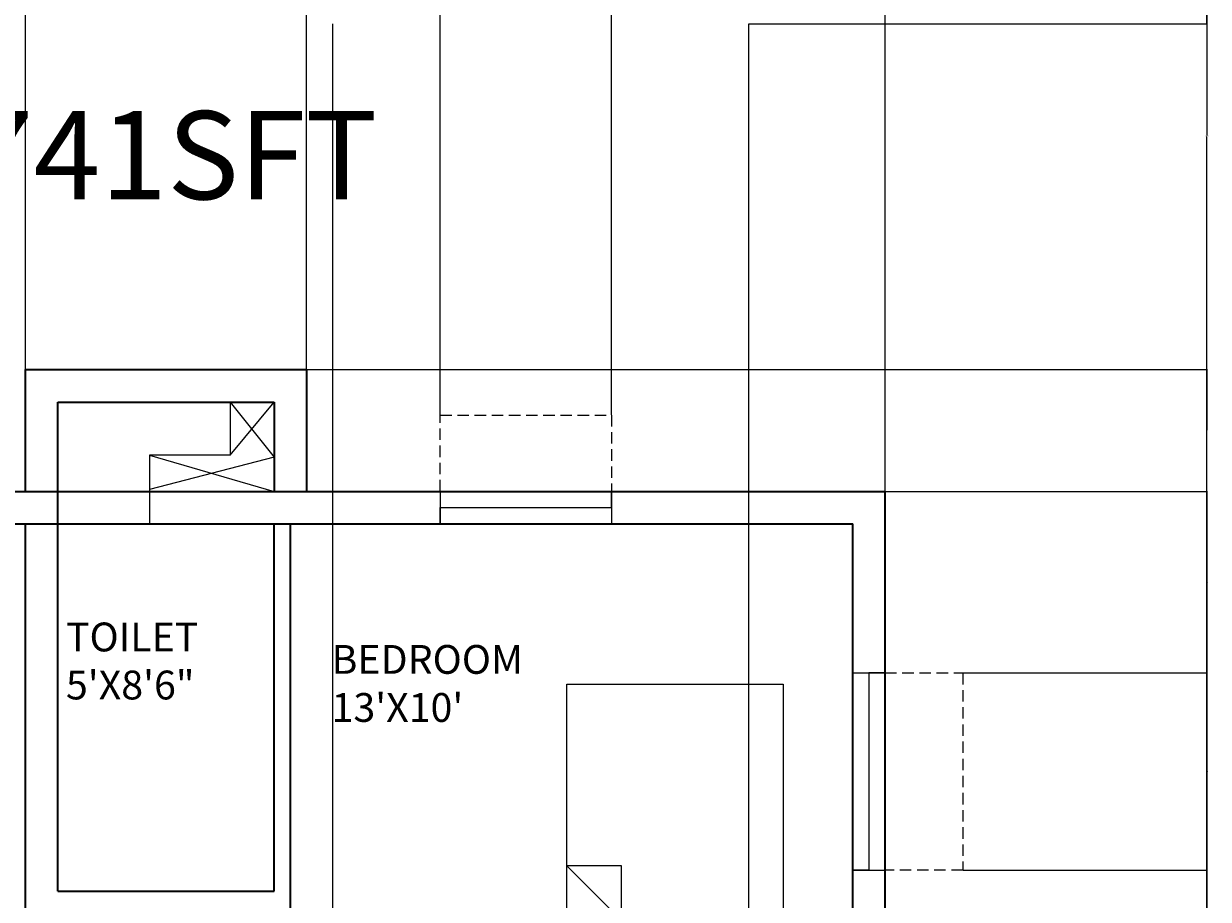
# Model space of a CAD drawing. Units: inches. Extents: x 276 to 912, y -567 to 621.
# Tile 4 of 7: x 583 to 912, y -178 to 65. Entities that reach past the tile are written whole.
import ezdxf

# ---------------------------------------------------------------- set-up
doc = ezdxf.new("R2010")
doc.units = ezdxf.units.IN
doc.linetypes.add('HIDDEN2', pattern=[4.7625, 3.175, -1.5875])
for name, color, linetype, lineweight in [('A-ANNO-DIMS', 2, 'Continuous', 18), ('A-ANNO-TEXT', 7, 'Continuous', 35), ('A-AREA-IDEN', 7, 'Continuous', 18), ('A-FLOR-OVHD', 8, 'HIDDEN2', 13), ('A-FLOR-SHFT', 8, 'Continuous', 18), ('A-FURN', 8, 'Continuous', 18), ('A-GLAZ', 4, 'Continuous', 18), ('A-WALL', 7, 'Continuous', 35)]:
    doc.layers.add(name, color=color, linetype=linetype, lineweight=lineweight)
doc.dimstyles.get("Standard").update_dxf_attribs({"dimtxt": 0.18, "dimasz": 0.18, "dimexe": 0.18, "dimexo": 0.0625, "dimgap": 0.09, "dimtad": 0, "dimtih": 1, "dimtoh": 1, "dimdec": 4, "dimzin": 0, "dimdsep": 46, "dimtxsty": 'Standard', "dimcen": 0.09, "dimadec": 0, "dimazin": 0, "dimtfac": 1, "dimtdec": 4, "dimtofl": 0, "dimtmove": 0, "dimatfit": 3, "dimfxl": 1, "dimtolj": 1, "dimtzin": 0, "dimarcsym": 0})

# ---------------------------------------------------------------- blocks, each defined once
blk = doc.blocks.new('Bed - Queen')
for p, q in [((0, -80.00003), (0, 0)), ((0, 0), (59.99999, 0)), ((59.99999, 0), (59.99999, -80.00003)), ((7.99999, -1.2), (28.79998, -1.2)), ((7.99999, -14.4), (7.99999, -1.2)), ((28.79998, -1.2), (28.79998, -14.4)), ((31.19999, -1.2), (51.99999, -1.2)), ((31.19999, -14.4), (31.19999, -1.2)), ((51.99999, -1.2), (51.99999, -16.4)), ((0, -14.4), (44.8, -14.4)), ((59.99999, -29.6), (44.8, -14.4)), ((44.8, -14.4), (44.8, -29.6)), ((51.99999, -16.4), (46.79936, -16.4)), ((44.8, -16.8), (0, -16.8)), ((44.8, -29.6), (59.99999, -29.6)), ((59.99999, -80.00003), (0, -80.00003))]:
    blk.add_line(p, q)
blk = doc.blocks.new('*D24')
at = {"layer": 'A-ANNO-DIMS', "color": 0, "lineweight": -2, "transparency": 16777216}
for p, q in [((333.082179, 103.255751), (333.082179, -553.223061)), ((854.209085, -327.604004), (854.209085, -553.223061)), ((333.262179, -553.043061), (593.255632, -553.043061)), ((854.029085, -553.043061), (594.035632, -553.043061))]:
    blk.add_line(p, q, dxfattribs=at)
at = {"layer": 'A-ANNO-DIMS', "color": 0, "transparency": 16777216}
for points in [[(333.262179, -553.013061), (333.262179, -553.073061), (333.082179, -553.043061)], [(854.029085, -553.013061), (854.029085, -553.073061), (854.209085, -553.043061)]]:
    blk.add_solid(points, dxfattribs=at)
at = {"layer": 'Defpoints', "color": 0, "transparency": 16777216}
for p in [(333.082179, 103.318251), (854.209085, -327.541504), (854.209085, -553.043061)]:
    blk.add_point(p, dxfattribs=at)
at = {"layer": 'A-ANNO-DIMS', "color": 0, "transparency": 16777216, "insert": (593.645632, -553.043061), "char_height": 0.18, "attachment_point": 5}
blk.add_mtext('\\A1;521.1', dxfattribs=at)
blk = doc.blocks.new('*D25')
at = {"layer": 'A-ANNO-DIMS', "color": 0, "lineweight": -2, "transparency": 16777216}
for p, q in [((478.5, 564.29), (911.39, 564.29)), ((911.21, 564.11), (911.21, 34.31)), ((911.21, -495.86), (911.21, 33.95)), ((582.98, -496.04), (911.39, -496.04))]:
    blk.add_line(p, q, dxfattribs=at)
at = {"layer": 'A-ANNO-DIMS', "color": 0, "transparency": 16777216}
for points in [[(911.18, 564.11), (911.24, 564.11), (911.21, 564.29)], [(911.18, -495.86), (911.24, -495.86), (911.21, -496.04)]]:
    blk.add_solid(points, dxfattribs=at)
at = {"layer": 'Defpoints', "color": 0, "transparency": 16777216}
for p in [(478.44, 564.29), (582.92, -496.04), (911.21, -496.04)]:
    blk.add_point(p, dxfattribs=at)
at = {"layer": 'A-ANNO-DIMS', "color": 0, "transparency": 16777216, "insert": (911.21, 34.13), "char_height": 0.18, "attachment_point": 5}
blk.add_mtext('\\A1;1060.3', dxfattribs=at)
blk = doc.blocks.new('*D33')
at = {"layer": 'A-ANNO-DIMS', "color": 0, "lineweight": -2, "transparency": 16777216}
for p, q in [((553.582179, 65.246155), (553.582179, -553.223061)), ((668.582179, 65.246155), (668.582179, -553.223061)), ((553.762179, -553.043061), (610.812179, -553.043061)), ((668.402179, -553.043061), (611.352179, -553.043061))]:
    blk.add_line(p, q, dxfattribs=at)
at = {"layer": 'A-ANNO-DIMS', "color": 0, "transparency": 16777216}
for points in [[(553.762179, -553.013061), (553.762179, -553.073061), (553.582179, -553.043061)], [(668.402179, -553.013061), (668.402179, -553.073061), (668.582179, -553.043061)]]:
    blk.add_solid(points, dxfattribs=at)
at = {"layer": 'Defpoints', "color": 0, "transparency": 16777216}
for p in [(553.582179, 65.308655), (668.582179, 65.308655), (668.582179, -553.043061)]:
    blk.add_point(p, dxfattribs=at)
at = {"layer": 'A-ANNO-DIMS', "color": 0, "transparency": 16777216, "insert": (611.082179, -553.043061), "char_height": 0.18, "attachment_point": 5}
blk.add_mtext('\\A1;115', dxfattribs=at)
blk = doc.blocks.new('*D34')
at = {"layer": 'A-ANNO-DIMS', "color": 0, "lineweight": -2, "transparency": 16777216}
for p, q in [((668.58, 65.25), (668.58, -553.22)), ((784, 65.25), (784, -553.22)), ((668.76, -553.04), (725.81, -553.04)), ((783.82, -553.04), (726.77, -553.04))]:
    blk.add_line(p, q, dxfattribs=at)
at = {"layer": 'A-ANNO-DIMS', "color": 0, "transparency": 16777216}
for points in [[(668.76, -553.01), (668.76, -553.07), (668.58, -553.04)], [(783.82, -553.01), (783.82, -553.07), (784, -553.04)]]:
    blk.add_solid(points, dxfattribs=at)
at = {"layer": 'Defpoints', "color": 0, "transparency": 16777216}
for p in [(668.58, 65.31), (784, 65.31), (784, -553.04)]:
    blk.add_point(p, dxfattribs=at)
at = {"layer": 'A-ANNO-DIMS', "color": 0, "transparency": 16777216, "insert": (726.29, -553.04), "char_height": 0.18, "attachment_point": 5}
blk.add_mtext('\\A1;115.42', dxfattribs=at)
blk = doc.blocks.new('*D35')
at = {"layer": 'A-ANNO-DIMS', "color": 0, "lineweight": -2, "transparency": 16777216}
for p, q in [((784.0623, 103.318251), (911.389085, 103.318251)), ((911.209085, 103.138251), (911.209085, 84.493453)), ((911.209085, 65.488655), (911.209085, 84.133453)), ((784.0623, 65.308655), (911.389085, 65.308655))]:
    blk.add_line(p, q, dxfattribs=at)
at = {"layer": 'A-ANNO-DIMS', "color": 0, "transparency": 16777216}
for points in [[(911.179085, 103.138251), (911.239085, 103.138251), (911.209085, 103.318251)], [(911.179085, 65.488655), (911.239085, 65.488655), (911.209085, 65.308655)]]:
    blk.add_solid(points, dxfattribs=at)
at = {"layer": 'Defpoints', "color": 0, "transparency": 16777216}
for p in [(783.9998, 103.318251), (911.209085, 103.318251), (783.9998, 65.308655)]:
    blk.add_point(p, dxfattribs=at)
at = {"layer": 'A-ANNO-DIMS', "color": 0, "transparency": 16777216, "insert": (911.209085, 84.313453), "char_height": 0.18, "attachment_point": 5}
blk.add_mtext('\\A1;38.01', dxfattribs=at)
blk = doc.blocks.new('*D54')
at = {"layer": 'A-ANNO-DIMS', "color": 0, "lineweight": -2, "transparency": 16777216}
for p, q in [((821.980989, -64.541504), (911.389085, -64.541504)), ((911.209085, -64.721504), (911.209085, -259.361504)), ((911.209085, -454.361504), (911.209085, -259.721504)), ((821.980989, -454.541504), (911.389085, -454.541504))]:
    blk.add_line(p, q, dxfattribs=at)
at = {"layer": 'A-ANNO-DIMS', "color": 0, "transparency": 16777216}
for points in [[(911.179085, -64.721504), (911.239085, -64.721504), (911.209085, -64.541504)], [(911.179085, -454.361504), (911.239085, -454.361504), (911.209085, -454.541504)]]:
    blk.add_solid(points, dxfattribs=at)
at = {"layer": 'Defpoints', "color": 0, "transparency": 16777216}
for p in [(821.918489, -64.541504), (821.918489, -454.541504), (911.209085, -454.541504)]:
    blk.add_point(p, dxfattribs=at)
at = {"layer": 'A-ANNO-DIMS', "color": 0, "transparency": 16777216, "insert": (911.209085, -259.541504), "char_height": 0.18, "attachment_point": 5}
blk.add_mtext('\\A1;390', dxfattribs=at)
blk = doc.blocks.new('*D59')
at = {"layer": 'A-ANNO-DIMS', "color": 0, "lineweight": -2, "transparency": 16777216}
for p, q in [((333.082179, -81.315568), (333.082179, 621.473746)), ((333.262179, 621.293746), (457.725334, 621.293746)), ((583.238489, 621.293746), (458.775334, 621.293746)), ((583.418489, -30.671128), (583.418489, 621.473746))]:
    blk.add_line(p, q, dxfattribs=at)
at = {"layer": 'A-ANNO-DIMS', "color": 0, "transparency": 16777216}
for points in [[(333.262179, 621.323746), (333.262179, 621.263746), (333.082179, 621.293746)], [(583.238489, 621.323746), (583.238489, 621.263746), (583.418489, 621.293746)]]:
    blk.add_solid(points, dxfattribs=at)
at = {"layer": 'Defpoints', "color": 0, "transparency": 16777216}
for p in [(583.418489, 621.293746), (583.418489, -30.733628), (333.082179, -81.378068)]:
    blk.add_point(p, dxfattribs=at)
at = {"layer": 'A-ANNO-DIMS', "color": 0, "transparency": 16777216, "insert": (458.250334, 621.293746), "char_height": 0.18, "attachment_point": 5}
blk.add_mtext('\\A1;250.34', dxfattribs=at)
blk = doc.blocks.new('*D60')
at = {"layer": 'A-ANNO-DIMS', "color": 0, "lineweight": -2, "transparency": 16777216}
for p, q in [((583.418489, -30.671128), (583.418489, 621.473746)), ((583.598489, 621.293746), (622.178489, 621.293746)), ((661.238489, 621.293746), (622.658489, 621.293746)), ((661.418489, -30.671128), (661.418489, 621.473746))]:
    blk.add_line(p, q, dxfattribs=at)
at = {"layer": 'A-ANNO-DIMS', "color": 0, "transparency": 16777216}
for points in [[(583.598489, 621.323746), (583.598489, 621.263746), (583.418489, 621.293746)], [(661.238489, 621.323746), (661.238489, 621.263746), (661.418489, 621.293746)]]:
    blk.add_solid(points, dxfattribs=at)
at = {"layer": 'Defpoints', "color": 0, "transparency": 16777216}
for p in [(661.418489, 621.293746), (583.418489, -30.733628), (661.418489, -30.733628)]:
    blk.add_point(p, dxfattribs=at)
at = {"layer": 'A-ANNO-DIMS', "color": 0, "transparency": 16777216, "insert": (622.418489, 621.293746), "char_height": 0.18, "attachment_point": 5}
blk.add_mtext('\\A1;78', dxfattribs=at)
blk = doc.blocks.new('*D61')
at = {"layer": 'A-ANNO-DIMS', "color": 0, "lineweight": -2, "transparency": 16777216}
for p, q in [((661.418489, -30.671128), (661.418489, 621.473746)), ((661.598489, 621.293746), (741.263489, 621.293746)), ((821.738489, 621.293746), (742.073489, 621.293746)), ((821.918489, -64.479004), (821.918489, 621.473746))]:
    blk.add_line(p, q, dxfattribs=at)
at = {"layer": 'A-ANNO-DIMS', "color": 0, "transparency": 16777216}
for points in [[(661.598489, 621.323746), (661.598489, 621.263746), (661.418489, 621.293746)], [(821.738489, 621.323746), (821.738489, 621.263746), (821.918489, 621.293746)]]:
    blk.add_solid(points, dxfattribs=at)
at = {"layer": 'Defpoints', "color": 0, "transparency": 16777216}
for p in [(821.918489, 621.293746), (661.418489, -30.733628), (821.918489, -64.541504)]:
    blk.add_point(p, dxfattribs=at)
at = {"layer": 'A-ANNO-DIMS', "color": 0, "transparency": 16777216, "insert": (741.668489, 621.293746), "char_height": 0.18, "attachment_point": 5}
blk.add_mtext('\\A1;160.5', dxfattribs=at)
blk = doc.blocks.new('*D62')
at = {"layer": 'A-ANNO-DIMS', "color": 0, "lineweight": -2, "transparency": 16777216}
for p, q in [((661.480989, -30.733628), (911.389085, -30.733628)), ((911.209085, -30.913628), (911.209085, -47.457566)), ((911.209085, -64.361504), (911.209085, -47.817566)), ((661.480989, -64.541504), (911.389085, -64.541504))]:
    blk.add_line(p, q, dxfattribs=at)
at = {"layer": 'A-ANNO-DIMS', "color": 0, "transparency": 16777216}
for points in [[(911.179085, -30.913628), (911.239085, -30.913628), (911.209085, -30.733628)], [(911.179085, -64.361504), (911.239085, -64.361504), (911.209085, -64.541504)]]:
    blk.add_solid(points, dxfattribs=at)
at = {"layer": 'Defpoints', "color": 0, "transparency": 16777216}
for p in [(661.418489, -30.733628), (661.418489, -64.541504), (911.209085, -64.541504)]:
    blk.add_point(p, dxfattribs=at)
at = {"layer": 'A-ANNO-DIMS', "color": 0, "transparency": 16777216, "insert": (911.209085, -47.637566), "char_height": 0.18, "attachment_point": 5}
blk.add_mtext('\\A1;33.81', dxfattribs=at)
blk = doc.blocks.new('*D72')
at = {"layer": 'A-ANNO-DIMS', "color": 0, "lineweight": -2, "transparency": 16777216}
for p, q in [((698.51, -43.28), (698.51, 621.47)), ((698.69, 621.29), (721.9, 621.29)), ((745.83, 621.29), (722.62, 621.29)), ((746.01, -43.28), (746.01, 621.47))]:
    blk.add_line(p, q, dxfattribs=at)
at = {"layer": 'A-ANNO-DIMS', "color": 0, "transparency": 16777216}
for points in [[(698.69, 621.32), (698.69, 621.26), (698.51, 621.29)], [(745.83, 621.32), (745.83, 621.26), (746.01, 621.29)]]:
    blk.add_solid(points, dxfattribs=at)
at = {"layer": 'Defpoints', "color": 0, "transparency": 16777216}
for p in [(746.01, 621.29), (698.51, -43.34), (746.01, -43.34)]:
    blk.add_point(p, dxfattribs=at)
at = {"layer": 'A-ANNO-DIMS', "color": 0, "transparency": 16777216, "insert": (722.26, 621.29), "char_height": 0.18, "attachment_point": 5}
blk.add_mtext('\\A1;47.5', dxfattribs=at)
blk = doc.blocks.new('*D73')
at = {"layer": 'A-ANNO-DIMS', "color": 0, "lineweight": -2, "transparency": 16777216}
for p, q in [((746.01, -43.28), (746.01, 621.47)), ((746.19, 621.29), (783.61, 621.29)), ((821.74, 621.29), (784.33, 621.29)), ((821.92, -64.48), (821.92, 621.47))]:
    blk.add_line(p, q, dxfattribs=at)
at = {"layer": 'A-ANNO-DIMS', "color": 0, "transparency": 16777216}
for points in [[(746.19, 621.32), (746.19, 621.26), (746.01, 621.29)], [(821.74, 621.32), (821.74, 621.26), (821.92, 621.29)]]:
    blk.add_solid(points, dxfattribs=at)
at = {"layer": 'Defpoints', "color": 0, "transparency": 16777216}
for p in [(821.92, 621.29), (746.01, -43.34), (821.92, -64.54)]:
    blk.add_point(p, dxfattribs=at)
at = {"layer": 'A-ANNO-DIMS', "color": 0, "transparency": 16777216, "insert": (783.97, 621.29), "char_height": 0.18, "attachment_point": 5}
blk.add_mtext('\\A1;75.9', dxfattribs=at)
blk = doc.blocks.new('*D76')
at = {"layer": 'A-ANNO-DIMS', "color": 0, "lineweight": -2, "transparency": 16777216}
for p, q in [((821.980989, -64.541504), (911.389085, -64.541504)), ((911.209085, -64.721504), (911.209085, -89.557289)), ((911.209085, -114.753074), (911.209085, -89.917289)), ((843.538697, -114.933074), (911.389085, -114.933074))]:
    blk.add_line(p, q, dxfattribs=at)
at = {"layer": 'A-ANNO-DIMS', "color": 0, "transparency": 16777216}
for points in [[(911.179085, -64.721504), (911.239085, -64.721504), (911.209085, -64.541504)], [(911.179085, -114.753074), (911.239085, -114.753074), (911.209085, -114.933074)]]:
    blk.add_solid(points, dxfattribs=at)
at = {"layer": 'Defpoints', "color": 0, "transparency": 16777216}
for p in [(821.918489, -64.541504), (843.476197, -114.933074), (911.209085, -114.933074)]:
    blk.add_point(p, dxfattribs=at)
at = {"layer": 'A-ANNO-DIMS', "color": 0, "transparency": 16777216, "insert": (911.209085, -89.737289), "char_height": 0.18, "attachment_point": 5}
blk.add_mtext('\\A1;50.39', dxfattribs=at)
blk = doc.blocks.new('*D77')
at = {"layer": 'A-ANNO-DIMS', "color": 0, "lineweight": -2, "transparency": 16777216}
for p, q in [((843.538697, -114.933074), (911.389085, -114.933074)), ((911.209085, -115.113074), (911.209085, -142.131)), ((911.209085, -169.508926), (911.209085, -142.491)), ((843.538697, -169.688926), (911.389085, -169.688926))]:
    blk.add_line(p, q, dxfattribs=at)
at = {"layer": 'A-ANNO-DIMS', "color": 0, "transparency": 16777216}
for points in [[(911.179085, -115.113074), (911.239085, -115.113074), (911.209085, -114.933074)], [(911.179085, -169.508926), (911.239085, -169.508926), (911.209085, -169.688926)]]:
    blk.add_solid(points, dxfattribs=at)
at = {"layer": 'Defpoints', "color": 0, "transparency": 16777216}
for p in [(843.476197, -114.933074), (843.476197, -169.688926), (911.209085, -169.688926)]:
    blk.add_point(p, dxfattribs=at)
at = {"layer": 'A-ANNO-DIMS', "color": 0, "transparency": 16777216, "insert": (911.209085, -142.311), "char_height": 0.18, "attachment_point": 5}
blk.add_mtext('\\A1;54.76', dxfattribs=at)

msp = doc.modelspace()

# ---------------------------------------------------------------- linework, layer by layer
at = {"layer": 'A-FLOR-OVHD'}
for p, q in [((698.5118, -64.5415), (698.5118, -43.3384)), ((698.5118, -43.3384), (746.0116, -43.3384)), ((746.0116, -43.3384), (746.0116, -64.5415)), ((821.9185, -114.9331), (843.4762, -114.9331)), ((843.4762, -114.9331), (843.4762, -169.6889)), ((843.4762, -169.6889), (821.9185, -169.6889))]:
    msp.add_line(p, q, dxfattribs=at)
at = {"layer": 'A-FLOR-SHFT'}
for p, q in [((640.1869, -39.7336), (640.1869, -54.4941)), ((640.1869, -54.4941), (652.4185, -39.7336)), ((640.1869, -39.7336), (652.4185, -55.0048)), ((628.5594, -54.4941), (617.8265, -54.4941)), ((617.8265, -54.4941), (617.8265, -73.5415)), ((617.8265, -54.4941), (652.4185, -64.5415)), ((652.4185, -55.0048), (617.8265, -64.0178)), ((640.1869, -54.4941), (628.5594, -54.4941))]:
    msp.add_line(p, q, dxfattribs=at)
at = {"layer": 'A-GLAZ'}
for p, q in [((698.5118, -64.5415), (698.5118, -73.5415)), ((746.0116, -69.0415), (746.0116, -64.5415)), ((746.0116, -64.5415), (746.0116, -73.5415)), ((698.5118, -73.5415), (698.5118, -69.0415)), ((698.5118, -69.0415), (746.0116, -69.0415)), ((812.9185, -114.9331), (821.9185, -114.9331)), ((821.9185, -114.9331), (817.4185, -114.9331)), ((817.4185, -114.9331), (817.4185, -169.6889)), ((817.4185, -169.6889), (812.9185, -169.6889)), ((812.9185, -169.6889), (821.9185, -169.6889))]:
    msp.add_line(p, q, dxfattribs=at)
at = {"layer": 'A-WALL'}
for p, q in [((583.4185, -30.7336), (661.4185, -30.7336)), ((583.4185, -64.5415), (583.4185, -30.7336)), ((661.4185, -30.7336), (661.4185, -64.5415)), ((592.4185, -64.5415), (592.4185, -39.7336)), ((592.4185, -39.7336), (652.4185, -39.7336)), ((652.4185, -39.7336), (652.4185, -64.5415)), ((342.0822, -64.5415), (821.9185, -64.5415)), ((592.4185, -73.5415), (592.4185, -64.5415)), ((821.9185, -238.9899), (821.9185, -64.5415)), ((342.0822, -73.5415), (812.9185, -73.5415)), ((583.4185, -207.5057), (583.4185, -73.5415)), ((592.4185, -175.5415), (592.4185, -73.5415)), ((652.4185, -175.5415), (652.4185, -73.5415)), ((656.9185, -207.5057), (656.9185, -73.5415)), ((812.9185, -198.5057), (812.9185, -73.5415)), ((592.4185, -175.5415), (652.4185, -175.5415))]:
    msp.add_line(p, q, dxfattribs=at)

# ---------------------------------------------------------------- block references
at = {"layer": 'A-FURN', "rotation": 180}
msp.add_blockref('Bed - Queen', (793.6066, -198.0637), dxfattribs=at)

# ---------------------------------------------------------------- texts
at = {"layer": 'A-ANNO-TEXT', "insert": (548.5415, 41.0446), "char_height": 24.49138, "attachment_point": 1}
msp.add_mtext_dynamic_manual_height_columns('{\\fTimes New Roman|b0|i0|c0|p18;1741SFT}', width=190.647076, gutter_width=38.2678, heights=[0], dxfattribs=at)
at = {"layer": 'A-AREA-IDEN', "char_height": 8, "attachment_point": 1}
for s, insert in [('{\\fTimes New Roman|b0|i0|c0|p18;TOILET\\P5\'X8\'6"}', (594.6445, -100.9592)), ("{\\fTimes New Roman|b0|i0|c0|p18;BEDROOM\\P13'X10'}", (668.3362, -107.1894))]:
    msp.add_mtext_dynamic_manual_height_columns(s, width=62.274017, gutter_width=12.5, heights=[0], dxfattribs=dict(at, insert=insert))

# ---------------------------------------------------------------- dimensions: what is measured, and where the dimension line sits
at = {"layer": 'A-ANNO-DIMS'}
for base, p1, p2, override, picture, middle in [((583.4185, 621.2937), (333.0822, -81.3781), (583.4185, -30.7336), {"dimdec": 2, "dimlfac": 1, "dimrnd": 0, "dimzin": 0, "dimdsep": 46, "dimlunit": 2}, '*D59', (458.2503, 621.2937)), ((661.4185, 621.2937), (583.4185, -30.7336), (661.4185, -30.7336), {"dimdec": 0, "dimlfac": 1, "dimrnd": 0, "dimzin": 0, "dimdsep": 46, "dimlunit": 2}, '*D60', (622.4185, 621.2937)), ((821.9185, 621.2937), (661.4185, -30.7336), (821.9185, -64.5415), {"dimdec": 1, "dimlfac": 1, "dimrnd": 0, "dimzin": 0, "dimdsep": 46, "dimlunit": 2}, '*D61', (741.6685, 621.2937)), ((746.0116, 621.2937), (698.5118, -43.3384), (746.0116, -43.3384), {"dimdec": 1, "dimlfac": 1, "dimrnd": 0, "dimzin": 0, "dimdsep": 46, "dimlunit": 2}, '*D72', (722.2617, 621.2937)), ((821.9185, 621.2937), (746.0116, -43.3384), (821.9185, -64.5415), {"dimdec": 1, "dimlfac": 1, "dimrnd": 0, "dimzin": 0, "dimdsep": 46, "dimlunit": 2}, '*D73', (783.9651, 621.2937)), ((854.2091, -553.0431), (333.0822, 103.3183), (854.2091, -327.5415), {"dimdec": 1, "dimlfac": 1, "dimrnd": 0, "dimzin": 0, "dimdsep": 46, "dimlunit": 2}, '*D24', (593.6456, -553.0431)), ((668.5822, -553.0431), (553.5822, 65.3087), (668.5822, 65.3087), {"dimdec": 0, "dimlfac": 1, "dimrnd": 0, "dimzin": 0, "dimdsep": 46, "dimlunit": 2}, '*D33', (611.0822, -553.0431)), ((783.9998, -553.0431), (668.5822, 65.3087), (783.9998, 65.3087), {"dimdec": 2, "dimlfac": 1, "dimrnd": 0, "dimzin": 0, "dimdsep": 46, "dimlunit": 2}, '*D34', (726.291, -553.0431))]:
    dim = msp.add_linear_dim(base=base, p1=p1, p2=p2, dimstyle='Standard', override=override, dxfattribs=at)
    dim.commit()
    dim.dimension.update_dxf_attribs({"geometry": picture, "text_midpoint": middle})
for base, p1, p2, override, picture, middle in [((911.2091, -496.0431), (478.4357, 564.2937), (582.9185, -496.0431), {"dimdec": 1, "dimlfac": 1, "dimrnd": 0, "dimzin": 0, "dimdsep": 46, "dimlunit": 2}, '*D25', (911.2091, 34.1253)), ((911.2091, 103.3183), (783.9998, 65.3087), (783.9998, 103.3183), {"dimdec": 2, "dimlfac": 1, "dimrnd": 0, "dimzin": 0, "dimdsep": 46, "dimlunit": 2}, '*D35', (911.2091, 84.3135)), ((911.2091, -64.5415), (661.4185, -30.7336), (661.4185, -64.5415), {"dimdec": 2, "dimlfac": 1, "dimrnd": 0, "dimzin": 0, "dimdsep": 46, "dimlunit": 2}, '*D62', (911.2091, -47.6376)), ((911.2091, -454.5415), (821.9185, -64.5415), (821.9185, -454.5415), {"dimdec": 0, "dimlfac": 1, "dimrnd": 0, "dimzin": 0, "dimdsep": 46, "dimlunit": 2}, '*D54', (911.2091, -259.5415)), ((911.2091, -114.9331), (821.9185, -64.5415), (843.4762, -114.9331), {"dimdec": 2, "dimlfac": 1, "dimrnd": 0, "dimzin": 0, "dimdsep": 46, "dimlunit": 2}, '*D76', (911.2091, -89.7373)), ((911.2091, -169.6889), (843.4762, -114.9331), (843.4762, -169.6889), {"dimdec": 2, "dimlfac": 1, "dimrnd": 0, "dimzin": 0, "dimdsep": 46, "dimlunit": 2}, '*D77', (911.2091, -142.311))]:
    dim = msp.add_linear_dim(base=base, p1=p1, p2=p2, angle=90, dimstyle='Standard', override=override, dxfattribs=at)
    dim.commit()
    dim.dimension.update_dxf_attribs({"geometry": picture, "text_midpoint": middle})

doc.saveas('drawing.dxf')
